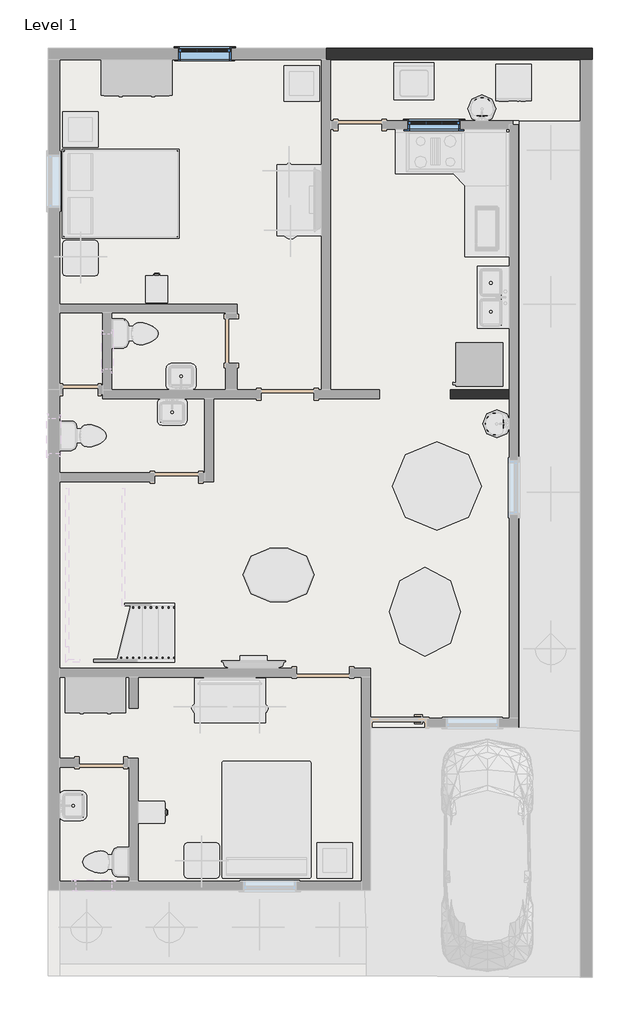
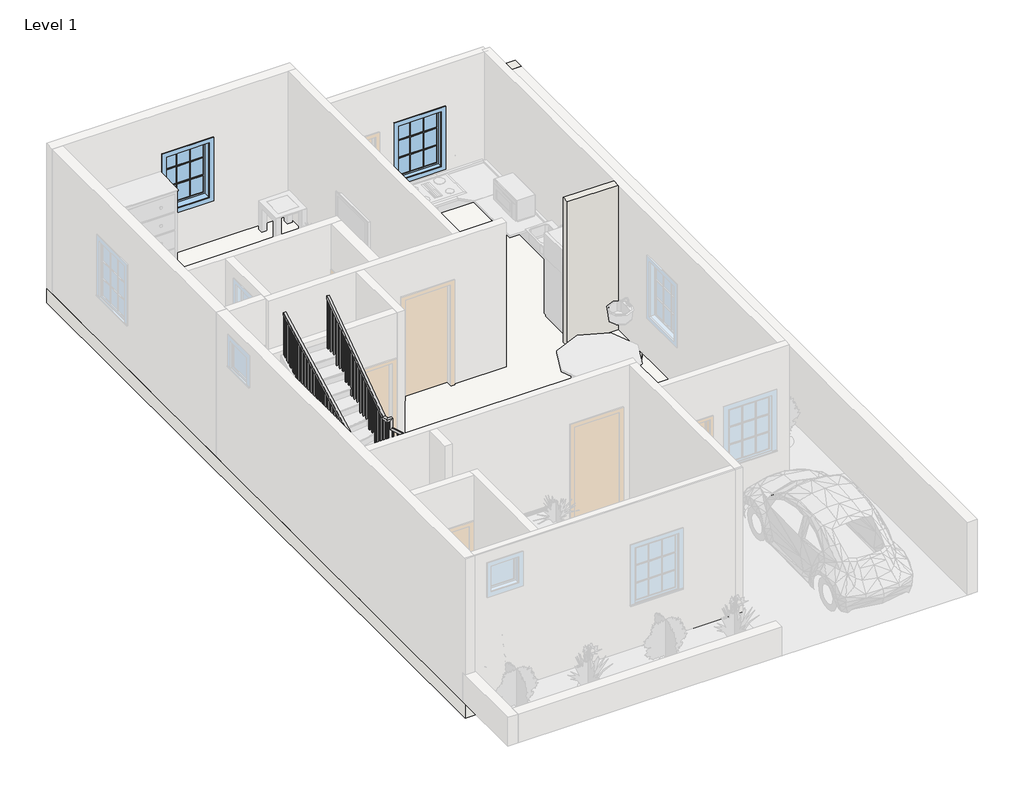
# One storey, part 2 of 3: 2 railings, 2 slabs, 2 walls, 2 windows.
"""IFC4 building model written with IfcOpenShell, lengths in millimetres."""

from ifc_helpers import new_model, si_unit, frame, origin, origin_with_axes, place, context, project, spatial, polyline, outline, extrude, faceted_brep, transform, mapped, element, save
from components import window_29c06734, window_5c190c7e

model = new_model("IFC4")

# Units and contexts
model_context = context("Model", 3, world=origin())
ifc_project = project(units=[si_unit("LENGTHUNIT", "METRE", prefix="MILLI")], contexts=[model_context])

# Site, building, storey
site = spatial("IfcSite", under=ifc_project)
building = spatial("IfcBuilding", under=site)
storey = spatial("IfcBuildingStorey", under=building, Name="Level 1", Elevation=0.0)

# Railings
placement = place(None, origin())
element("IfcRailing", 1, ObjectType="Handrail - Rectangular", at=placement, inside=storey, context=model_context, shape_type="SolidModel", body=[
    faceted_brep([(-12359.4290643, 4743.353629, 1682.9646102), (-12359.4290643, 4743.353629, 1615.1075334), (-12359.4290643, 4794.153629, 1615.1075334), (-12359.4290643, 4794.153629, 1682.9646102), (-13187.1660538, 4743.353629, 2416.0047843), (-13237.9660538, 4743.353629, 2393.1359601), (-13237.9660538, 4794.153629, 2393.1359601), (-13187.1660538, 4794.153629, 2416.0047843), (-13187.1660538, 4743.353629, 2625.457216), (-13237.9660538, 4743.353629, 2574.657216), (-13237.9660538, 4794.153629, 2574.657216), (-13187.1660538, 4794.153629, 2625.457216), (-13314.1660538, 4743.353629, 2625.457216), (-13314.1660538, 4743.353629, 2574.657216), (-13263.3660538, 4794.153629, 2574.657216), (-13263.3660538, 4794.153629, 2625.457216), (-13314.1660538, 4870.353629, 2625.457216), (-13314.1660538, 4886.3832649, 2574.657216), (-13263.3660538, 4886.3832649, 2574.657216), (-13263.3660538, 4870.353629, 2625.457216), (-13314.1660538, 6815.6906185, 3988.8904479), (-13263.3660538, 6815.6906185, 3988.8904479), (-13263.3660538, 6815.6906185, 3926.8557166), (-13314.1660538, 6815.6906185, 3926.8557166)], [[[0, 1, 2, 3]], [[1, 0, 4, 5]], [[2, 1, 5, 6]], [[3, 2, 6, 7]], [[0, 3, 7, 4]], [[5, 4, 8, 9]], [[6, 5, 9, 10]], [[7, 6, 10, 11]], [[4, 7, 11, 8]], [[9, 8, 12, 13]], [[10, 9, 13, 14]], [[11, 10, 14, 15]], [[8, 11, 15, 12]], [[13, 12, 16, 17]], [[14, 13, 17, 18]], [[15, 14, 18, 19]], [[12, 15, 19, 16]], [[20, 21, 22, 23]], [[17, 16, 20, 23]], [[18, 17, 23, 22]], [[19, 18, 22, 21]], [[16, 19, 21, 20]]]),
    extrude(outline(polyline([(6791.228629, 3909.7109805), (6810.278629, 3923.0626019), (6810.278629, 2878.6666667), (6791.228629, 2878.6666667), (6791.228629, 3909.7109805)])), frame((-13298.2910538, 0.0, 0.0), z_axis=(1.0, 0.0, 0.0), x_axis=(0.0, 1.0, 0.0)), (0.0, 0.0, 1.0), 19.05),
    extrude(outline(polyline([(6689.628629, 3838.5023328), (6708.678629, 3851.8539542), (6708.678629, 2878.6666667), (6689.628629, 2878.6666667), (6689.628629, 3838.5023328)])), frame((-13298.2910538, 0.0, 0.0), z_axis=(1.0, 0.0, 0.0), x_axis=(0.0, 1.0, 0.0)), (0.0, 0.0, 1.0), 19.05),
    extrude(outline(polyline([(6588.028629, 3767.3719643), (6607.078629, 3780.7235858), (6607.078629, 2878.6666667), (6588.028629, 2878.6666667), (6588.028629, 3767.3719643)])), frame((-13298.2910538, 0.0, 0.0), z_axis=(1.0, 0.0, 0.0), x_axis=(0.0, 1.0, 0.0)), (0.0, 0.0, 1.0), 19.05),
    extrude(outline(polyline([(6486.428629, 3696.1633166), (6505.478629, 3709.514938), (6505.478629, 2709.3333333), (6486.428629, 2709.3333333), (6486.428629, 3696.1633166)])), frame((-13298.2910538, 0.0, 0.0), z_axis=(1.0, 0.0, 0.0), x_axis=(0.0, 1.0, 0.0)), (0.0, 0.0, 1.0), 19.05),
    extrude(outline(polyline([(6384.828629, 3624.9546689), (6403.878629, 3638.3062903), (6403.878629, 2709.3333333), (6384.828629, 2709.3333333), (6384.828629, 3624.9546689)])), frame((-13298.2910538, 0.0, 0.0), z_axis=(1.0, 0.0, 0.0), x_axis=(0.0, 1.0, 0.0)), (0.0, 0.0, 1.0), 19.05),
    extrude(outline(polyline([(6283.228629, 3553.667742), (6302.278629, 3567.0193634), (6302.278629, 2709.3333333), (6283.228629, 2709.3333333), (6283.228629, 3553.667742)])), frame((-13298.2910538, 0.0, 0.0), z_axis=(1.0, 0.0, 0.0), x_axis=(0.0, 1.0, 0.0)), (0.0, 0.0, 1.0), 19.05),
    extrude(outline(polyline([(6181.628629, 3482.5373735), (6200.678629, 3495.8889949), (6200.678629, 2540.0), (6181.628629, 2540.0), (6181.628629, 3482.5373735)])), frame((-13298.2910538, 0.0, 0.0), z_axis=(1.0, 0.0, 0.0), x_axis=(0.0, 1.0, 0.0)), (0.0, 0.0, 1.0), 19.05),
    extrude(outline(polyline([(6080.028629, 3411.2504466), (6099.078629, 3424.602068), (6099.078629, 2540.0), (6080.028629, 2540.0), (6080.028629, 3411.2504466)])), frame((-13298.2910538, 0.0, 0.0), z_axis=(1.0, 0.0, 0.0), x_axis=(0.0, 1.0, 0.0)), (0.0, 0.0, 1.0), 19.05),
    extrude(outline(polyline([(5978.428629, 3340.1200781), (5997.478629, 3353.4716995), (5997.478629, 2370.6666667), (5978.428629, 2370.6666667), (5978.428629, 3340.1200781)])), frame((-13298.2910538, 0.0, 0.0), z_axis=(1.0, 0.0, 0.0), x_axis=(0.0, 1.0, 0.0)), (0.0, 0.0, 1.0), 19.05),
    extrude(outline(polyline([(5876.828629, 3268.8331511), (5895.878629, 3282.1847726), (5895.878629, 2370.6666667), (5876.828629, 2370.6666667), (5876.828629, 3268.8331511)])), frame((-13298.2910538, 0.0, 0.0), z_axis=(1.0, 0.0, 0.0), x_axis=(0.0, 1.0, 0.0)), (0.0, 0.0, 1.0), 19.05),
    extrude(outline(polyline([(5775.228629, 3197.6245034), (5794.278629, 3210.9761249), (5794.278629, 2370.6666667), (5775.228629, 2370.6666667), (5775.228629, 3197.6245034)])), frame((-13298.2910538, 0.0, 0.0), z_axis=(1.0, 0.0, 0.0), x_axis=(0.0, 1.0, 0.0)), (0.0, 0.0, 1.0), 19.05),
    extrude(outline(polyline([(5673.628629, 3126.494135), (5692.678629, 3139.8457564), (5692.678629, 2201.3333333), (5673.628629, 2201.3333333), (5673.628629, 3126.494135)])), frame((-13298.2910538, 0.0, 0.0), z_axis=(1.0, 0.0, 0.0), x_axis=(0.0, 1.0, 0.0)), (0.0, 0.0, 1.0), 19.05),
    extrude(outline(polyline([(5572.028629, 3055.207208), (5591.078629, 3068.5588295), (5591.078629, 2201.3333333), (5572.028629, 2201.3333333), (5572.028629, 3055.207208)])), frame((-13298.2910538, 0.0, 0.0), z_axis=(1.0, 0.0, 0.0), x_axis=(0.0, 1.0, 0.0)), (0.0, 0.0, 1.0), 19.05),
    extrude(outline(polyline([(5470.428629, 2983.9985603), (5489.478629, 2997.3501818), (5489.478629, 2201.3333333), (5470.428629, 2201.3333333), (5470.428629, 2983.9985603)])), frame((-13298.2910538, 0.0, 0.0), z_axis=(1.0, 0.0, 0.0), x_axis=(0.0, 1.0, 0.0)), (0.0, 0.0, 1.0), 19.05),
    extrude(outline(polyline([(5368.828629, 2912.7899126), (5387.878629, 2926.1415341), (5387.878629, 2032.0), (5368.828629, 2032.0), (5368.828629, 2912.7899126)])), frame((-13298.2910538, 0.0, 0.0), z_axis=(1.0, 0.0, 0.0), x_axis=(0.0, 1.0, 0.0)), (0.0, 0.0, 1.0), 19.05),
    extrude(outline(polyline([(5267.228629, 2841.5812649), (5286.278629, 2854.9328864), (5286.278629, 2032.0), (5267.228629, 2032.0), (5267.228629, 2841.5812649)])), frame((-13298.2910538, 0.0, 0.0), z_axis=(1.0, 0.0, 0.0), x_axis=(0.0, 1.0, 0.0)), (0.0, 0.0, 1.0), 19.05),
    extrude(outline(polyline([(5165.628629, 2770.4508964), (5184.678629, 2783.8025179), (5184.678629, 1862.6666667), (5165.628629, 1862.6666667), (5165.628629, 2770.4508964)])), frame((-13298.2910538, 0.0, 0.0), z_axis=(1.0, 0.0, 0.0), x_axis=(0.0, 1.0, 0.0)), (0.0, 0.0, 1.0), 19.05),
    extrude(outline(polyline([(5064.028629, 2699.1639695), (5083.078629, 2712.515591), (5083.078629, 1862.6666667), (5064.028629, 1862.6666667), (5064.028629, 2699.1639695)])), frame((-13298.2910538, 0.0, 0.0), z_axis=(1.0, 0.0, 0.0), x_axis=(0.0, 1.0, 0.0)), (0.0, 0.0, 1.0), 19.05),
    extrude(outline(polyline([(4962.428629, 2628.033601), (4981.478629, 2641.3852225), (4981.478629, 1693.3333333), (4962.428629, 1693.3333333), (4962.428629, 2628.033601)])), frame((-13298.2910538, 0.0, 0.0), z_axis=(1.0, 0.0, 0.0), x_axis=(0.0, 1.0, 0.0)), (0.0, 0.0, 1.0), 19.05),
    extrude(outline(polyline([(-13279.2410538, 4860.828629), (-13298.2910538, 4860.828629), (-13298.2910538, 4879.878629), (-13279.2410538, 4879.878629), (-13279.2410538, 4860.828629)])), frame((0.0, 0.0, 1693.3333333), z_axis=(0.0, 0.0, 1.0), x_axis=(1.0, 0.0, 0.0)), (0.0, 0.0, 1.0), 881.3238827),
    extrude(outline(polyline([(-13264.3040643, 4778.278629), (-13264.3040643, 4759.228629), (-13283.3540643, 4759.228629), (-13283.3540643, 4778.278629), (-13264.3040643, 4778.278629)])), frame((0.0, 0.0, 1524.0), z_axis=(0.0, 0.0, 1.0), x_axis=(1.0, 0.0, 0.0)), (0.0, 0.0, 1.0), 1050.657216),
    extrude(outline(polyline([(2326.484279, -13162.7040643), (2343.3548737, -13181.7540643), (1354.6666667, -13181.7540643), (1354.6666667, -13162.7040643), (2326.484279, -13162.7040643)])), frame((0.0, 4759.228629, 0.0), z_axis=(0.0, 1.0, 0.0), x_axis=(0.0, 0.0, 1.0)), (0.0, 0.0, 1.0), 19.05),
    extrude(outline(polyline([(2236.5077736, -13061.1040643), (2253.3783684, -13080.1540643), (1185.3333333, -13080.1540643), (1185.3333333, -13061.1040643), (2236.5077736, -13061.1040643)])), frame((0.0, 4759.228629, 0.0), z_axis=(0.0, 1.0, 0.0), x_axis=(0.0, 0.0, 1.0)), (0.0, 0.0, 1.0), 19.05),
    extrude(outline(polyline([(2146.5312682, -12959.5040643), (2163.401863, -12978.5540643), (1185.3333333, -12978.5540643), (1185.3333333, -12959.5040643), (2146.5312682, -12959.5040643)])), frame((0.0, 4759.228629, 0.0), z_axis=(0.0, 1.0, 0.0), x_axis=(0.0, 0.0, 1.0)), (0.0, 0.0, 1.0), 19.05),
    extrude(outline(polyline([(2056.5547629, -12857.9040643), (2073.4253576, -12876.9540643), (1016.0, -12876.9540643), (1016.0, -12857.9040643), (2056.5547629, -12857.9040643)])), frame((0.0, 4759.228629, 0.0), z_axis=(0.0, 1.0, 0.0), x_axis=(0.0, 0.0, 1.0)), (0.0, 0.0, 1.0), 19.05),
    extrude(outline(polyline([(1966.5782575, -12756.3040643), (1983.4488522, -12775.3540643), (1016.0, -12775.3540643), (1016.0, -12756.3040643), (1966.5782575, -12756.3040643)])), frame((0.0, 4759.228629, 0.0), z_axis=(0.0, 1.0, 0.0), x_axis=(0.0, 0.0, 1.0)), (0.0, 0.0, 1.0), 19.05),
    extrude(outline(polyline([(1876.6017521, -12654.7040643), (1893.4723469, -12673.7540643), (1016.0, -12673.7540643), (1016.0, -12654.7040643), (1876.6017521, -12654.7040643)])), frame((0.0, 4759.228629, 0.0), z_axis=(0.0, 1.0, 0.0), x_axis=(0.0, 0.0, 1.0)), (0.0, 0.0, 1.0), 19.05),
    extrude(outline(polyline([(1786.6252467, -12553.1040643), (1803.4958415, -12572.1540643), (846.6666667, -12572.1540643), (846.6666667, -12553.1040643), (1786.6252467, -12553.1040643)])), frame((0.0, 4759.228629, 0.0), z_axis=(0.0, 1.0, 0.0), x_axis=(0.0, 0.0, 1.0)), (0.0, 0.0, 1.0), 19.05),
    extrude(outline(polyline([(1696.6487414, -12451.5040643), (1713.5193361, -12470.5540643), (846.6666667, -12470.5540643), (846.6666667, -12451.5040643), (1696.6487414, -12451.5040643)])), frame((0.0, 4759.228629, 0.0), z_axis=(0.0, 1.0, 0.0), x_axis=(0.0, 0.0, 1.0)), (0.0, 0.0, 1.0), 19.05),
    extrude(outline(polyline([(-13279.2410538, 4759.228629), (-13298.2910538, 4759.228629), (-13298.2910538, 4778.278629), (-13279.2410538, 4778.278629), (-13279.2410538, 4759.228629)])), frame((0.0, 0.0, 1524.0), z_axis=(0.0, 0.0, 1.0), x_axis=(1.0, 0.0, 0.0)), (0.0, 0.0, 1.0), 1050.657216),
    extrude(outline(polyline([(6796.6406185, 3913.5040952), (6815.6906185, 3926.8557166), (6815.6906185, 2878.6666667), (6796.6406185, 2878.6666667), (6796.6406185, 3913.5040952)])), frame((-13298.2910538, 0.0, 0.0), z_axis=(1.0, 0.0, 0.0), x_axis=(0.0, 1.0, 0.0)), (0.0, 0.0, 1.0), 19.05),
    extrude(outline(polyline([(1615.1075334, -12359.4290643), (1631.9781281, -12378.4790643), (846.6666667, -12378.4790643), (846.6666667, -12359.4290643), (1615.1075334, -12359.4290643)])), frame((0.0, 4759.228629, 0.0), z_axis=(0.0, 1.0, 0.0), x_axis=(0.0, 0.0, 1.0)), (0.0, 0.0, 1.0), 19.05),
])
element("IfcRailing", 2, ObjectType="Handrail - Rectangular", at=placement, inside=storey, context=model_context, shape_type="SolidModel", body=[
    faceted_brep([(-12359.4290643, 3879.753629, 1807.8545254), (-12359.4290643, 3879.753629, 1752.3830665), (-12359.4290643, 3930.553629, 1752.3830665), (-12359.4290643, 3930.553629, 1807.8545254), (-13956.7820986, 3879.753629, 2508.4571941), (-13967.4328846, 3879.753629, 2457.6571941), (-13967.4328846, 3930.553629, 2457.6571941), (-13956.7820986, 3930.553629, 2508.4571941), (-14177.7660538, 3879.753629, 2508.4571941), (-14177.7660538, 3879.753629, 2457.6571941), (-14126.9660538, 3930.553629, 2457.6571941), (-14126.9660538, 3930.553629, 2508.4571941), (-14177.7660538, 4069.8569729, 2508.4571941), (-14177.7660538, 4082.2933675, 2457.6571941), (-14126.9660538, 4082.2933675, 2457.6571941), (-14126.9660538, 4069.8569729, 2508.4571941), (-14177.7660538, 6815.6906185, 3938.588476), (-14126.9660538, 6815.6906185, 3938.588476), (-14126.9660538, 6815.6906185, 3881.3111437), (-14177.7660538, 6815.6906185, 3881.3111437)], [[[0, 1, 2, 3]], [[1, 0, 4, 5]], [[2, 1, 5, 6]], [[3, 2, 6, 7]], [[0, 3, 7, 4]], [[5, 4, 8, 9]], [[6, 5, 9, 10]], [[7, 6, 10, 11]], [[4, 7, 11, 8]], [[9, 8, 12, 13]], [[10, 9, 13, 14]], [[11, 10, 14, 15]], [[8, 11, 15, 12]], [[16, 17, 18, 19]], [[13, 12, 16, 19]], [[14, 13, 19, 18]], [[15, 14, 18, 17]], [[12, 15, 17, 16]]]),
    extrude(outline(polyline([(6822.5819729, 3884.8947365), (6822.5819729, 2878.6666667), (6803.5319729, 2878.6666667), (6803.5319729, 3874.9727949), (6822.5819729, 3884.8947365)])), frame((-14161.8910538, 0.0, 0.0), z_axis=(1.0, 0.0, 0.0), x_axis=(0.0, 1.0, 0.0)), (0.0, 0.0, 1.0), 19.05),
    extrude(outline(polyline([(6720.9819729, 3831.9777149), (6720.9819729, 2878.6666667), (6701.9319729, 2878.6666667), (6701.9319729, 3822.0557734), (6720.9819729, 3831.9777149)])), frame((-14161.8910538, 0.0, 0.0), z_axis=(1.0, 0.0, 0.0), x_axis=(0.0, 1.0, 0.0)), (0.0, 0.0, 1.0), 19.05),
    extrude(outline(polyline([(6619.3819729, 3779.0663717), (6619.3819729, 2878.6666667), (6600.3319729, 2878.6666667), (6600.3319729, 3769.1444302), (6619.3819729, 3779.0663717)])), frame((-14161.8910538, 0.0, 0.0), z_axis=(1.0, 0.0, 0.0), x_axis=(0.0, 1.0, 0.0)), (0.0, 0.0, 1.0), 19.05),
    extrude(outline(polyline([(6517.7819729, 3726.1436718), (6517.7819729, 2709.3333333), (6498.7319729, 2709.3333333), (6498.7319729, 3716.2217303), (6517.7819729, 3726.1436718)])), frame((-14161.8910538, 0.0, 0.0), z_axis=(1.0, 0.0, 0.0), x_axis=(0.0, 1.0, 0.0)), (0.0, 0.0, 1.0), 19.05),
    extrude(outline(polyline([(6416.1819729, 3673.2266502), (6416.1819729, 2709.3333333), (6397.1319729, 2709.3333333), (6397.1319729, 3663.3047087), (6416.1819729, 3673.2266502)])), frame((-14161.8910538, 0.0, 0.0), z_axis=(1.0, 0.0, 0.0), x_axis=(0.0, 1.0, 0.0)), (0.0, 0.0, 1.0), 19.05),
    extrude(outline(polyline([(6314.5819729, 3620.315307), (6314.5819729, 2709.3333333), (6295.5319729, 2709.3333333), (6295.5319729, 3610.3933655), (6314.5819729, 3620.315307)])), frame((-14161.8910538, 0.0, 0.0), z_axis=(1.0, 0.0, 0.0), x_axis=(0.0, 1.0, 0.0)), (0.0, 0.0, 1.0), 19.05),
    extrude(outline(polyline([(6212.9819729, 3567.3926071), (6212.9819729, 2540.0), (6193.9319729, 2540.0), (6193.9319729, 3557.4706656), (6212.9819729, 3567.3926071)])), frame((-14161.8910538, 0.0, 0.0), z_axis=(1.0, 0.0, 0.0), x_axis=(0.0, 1.0, 0.0)), (0.0, 0.0, 1.0), 19.05),
    extrude(outline(polyline([(6111.3819729, 3514.4755855), (6111.3819729, 2540.0), (6092.3319729, 2540.0), (6092.3319729, 3504.553644), (6111.3819729, 3514.4755855)])), frame((-14161.8910538, 0.0, 0.0), z_axis=(1.0, 0.0, 0.0), x_axis=(0.0, 1.0, 0.0)), (0.0, 0.0, 1.0), 19.05),
    extrude(outline(polyline([(6009.7819729, 3461.558564), (6009.7819729, 2540.0), (5990.7319729, 2540.0), (5990.7319729, 3451.6366224), (6009.7819729, 3461.558564)])), frame((-14161.8910538, 0.0, 0.0), z_axis=(1.0, 0.0, 0.0), x_axis=(0.0, 1.0, 0.0)), (0.0, 0.0, 1.0), 19.05),
    extrude(outline(polyline([(5908.1819729, 3408.6415424), (5908.1819729, 2370.6666667), (5889.1319729, 2370.6666667), (5889.1319729, 3398.7196009), (5908.1819729, 3408.6415424)])), frame((-14161.8910538, 0.0, 0.0), z_axis=(1.0, 0.0, 0.0), x_axis=(0.0, 1.0, 0.0)), (0.0, 0.0, 1.0), 19.05),
    extrude(outline(polyline([(5806.5819729, 3355.7245208), (5806.5819729, 2370.6666667), (5787.5319729, 2370.6666667), (5787.5319729, 3345.8025793), (5806.5819729, 3355.7245208)])), frame((-14161.8910538, 0.0, 0.0), z_axis=(1.0, 0.0, 0.0), x_axis=(0.0, 1.0, 0.0)), (0.0, 0.0, 1.0), 19.05),
    extrude(outline(polyline([(5704.9819729, 3302.8131776), (5704.9819729, 2370.6666667), (5685.9319729, 2370.6666667), (5685.9319729, 3292.8912361), (5704.9819729, 3302.8131776)])), frame((-14161.8910538, 0.0, 0.0), z_axis=(1.0, 0.0, 0.0), x_axis=(0.0, 1.0, 0.0)), (0.0, 0.0, 1.0), 19.05),
    extrude(outline(polyline([(5603.3819729, 3249.8961561), (5603.3819729, 2201.3333333), (5584.3319729, 2201.3333333), (5584.3319729, 3239.9742145), (5603.3819729, 3249.8961561)])), frame((-14161.8910538, 0.0, 0.0), z_axis=(1.0, 0.0, 0.0), x_axis=(0.0, 1.0, 0.0)), (0.0, 0.0, 1.0), 19.05),
    extrude(outline(polyline([(5501.7819729, 3196.9791345), (5501.7819729, 2201.3333333), (5482.7319729, 2201.3333333), (5482.7319729, 3187.057193), (5501.7819729, 3196.9791345)])), frame((-14161.8910538, 0.0, 0.0), z_axis=(1.0, 0.0, 0.0), x_axis=(0.0, 1.0, 0.0)), (0.0, 0.0, 1.0), 19.05),
    extrude(outline(polyline([(5400.1819729, 3144.062113), (5400.1819729, 2201.3333333), (5381.1319729, 2201.3333333), (5381.1319729, 3134.1401714), (5400.1819729, 3144.062113)])), frame((-14161.8910538, 0.0, 0.0), z_axis=(1.0, 0.0, 0.0), x_axis=(0.0, 1.0, 0.0)), (0.0, 0.0, 1.0), 19.05),
    extrude(outline(polyline([(5298.5819729, 3091.1450914), (5298.5819729, 2032.0), (5279.5319729, 2032.0), (5279.5319729, 3081.2231498), (5298.5819729, 3091.1450914)])), frame((-14161.8910538, 0.0, 0.0), z_axis=(1.0, 0.0, 0.0), x_axis=(0.0, 1.0, 0.0)), (0.0, 0.0, 1.0), 19.05),
    extrude(outline(polyline([(5196.9819729, 3038.2280698), (5196.9819729, 2032.0), (5177.9319729, 2032.0), (5177.9319729, 3028.3061283), (5196.9819729, 3038.2280698)])), frame((-14161.8910538, 0.0, 0.0), z_axis=(1.0, 0.0, 0.0), x_axis=(0.0, 1.0, 0.0)), (0.0, 0.0, 1.0), 19.05),
    extrude(outline(polyline([(5095.3819729, 2985.3110483), (5095.3819729, 2032.0), (5076.3319729, 2032.0), (5076.3319729, 2975.3891067), (5095.3819729, 2985.3110483)])), frame((-14161.8910538, 0.0, 0.0), z_axis=(1.0, 0.0, 0.0), x_axis=(0.0, 1.0, 0.0)), (0.0, 0.0, 1.0), 19.05),
    extrude(outline(polyline([(4993.7819729, 2932.3940267), (4993.7819729, 1862.6666667), (4974.7319729, 1862.6666667), (4974.7319729, 2922.4720852), (4993.7819729, 2932.3940267)])), frame((-14161.8910538, 0.0, 0.0), z_axis=(1.0, 0.0, 0.0), x_axis=(0.0, 1.0, 0.0)), (0.0, 0.0, 1.0), 19.05),
    extrude(outline(polyline([(4892.1819729, 2879.4770051), (4892.1819729, 1862.6666667), (4873.1319729, 1862.6666667), (4873.1319729, 2869.5550636), (4892.1819729, 2879.4770051)])), frame((-14161.8910538, 0.0, 0.0), z_axis=(1.0, 0.0, 0.0), x_axis=(0.0, 1.0, 0.0)), (0.0, 0.0, 1.0), 19.05),
    extrude(outline(polyline([(4790.5819729, 2826.5599836), (4790.5819729, 1862.6666667), (4771.5319729, 1862.6666667), (4771.5319729, 2816.638042), (4790.5819729, 2826.5599836)])), frame((-14161.8910538, 0.0, 0.0), z_axis=(1.0, 0.0, 0.0), x_axis=(0.0, 1.0, 0.0)), (0.0, 0.0, 1.0), 19.05),
    extrude(outline(polyline([(4688.9819729, 2773.642962), (4688.9819729, 1693.3333333), (4669.9319729, 1693.3333333), (4669.9319729, 2763.7210205), (4688.9819729, 2773.642962)])), frame((-14161.8910538, 0.0, 0.0), z_axis=(1.0, 0.0, 0.0), x_axis=(0.0, 1.0, 0.0)), (0.0, 0.0, 1.0), 19.05),
    extrude(outline(polyline([(4587.3819729, 2720.7259404), (4587.3819729, 1693.3333333), (4568.3319729, 1693.3333333), (4568.3319729, 2710.8039989), (4587.3819729, 2720.7259404)])), frame((-14161.8910538, 0.0, 0.0), z_axis=(1.0, 0.0, 0.0), x_axis=(0.0, 1.0, 0.0)), (0.0, 0.0, 1.0), 19.05),
    extrude(outline(polyline([(4485.7819729, 2667.8089189), (4485.7819729, 1693.3333333), (4466.7319729, 1693.3333333), (4466.7319729, 2657.8869773), (4485.7819729, 2667.8089189)])), frame((-14161.8910538, 0.0, 0.0), z_axis=(1.0, 0.0, 0.0), x_axis=(0.0, 1.0, 0.0)), (0.0, 0.0, 1.0), 19.05),
    extrude(outline(polyline([(4384.1819729, 2614.8918973), (4384.1819729, 1693.3333333), (4365.1319729, 1693.3333333), (4365.1319729, 2604.9699558), (4384.1819729, 2614.8918973)])), frame((-14161.8910538, 0.0, 0.0), z_axis=(1.0, 0.0, 0.0), x_axis=(0.0, 1.0, 0.0)), (0.0, 0.0, 1.0), 19.05),
    extrude(outline(polyline([(4282.5819729, 2561.9748757), (4282.5819729, 1524.0), (4263.5319729, 1524.0), (4263.5319729, 2552.0529342), (4282.5819729, 2561.9748757)])), frame((-14161.8910538, 0.0, 0.0), z_axis=(1.0, 0.0, 0.0), x_axis=(0.0, 1.0, 0.0)), (0.0, 0.0, 1.0), 19.05),
    extrude(outline(polyline([(4180.9819729, 2509.0578542), (4180.9819729, 1524.0), (4161.9319729, 1524.0), (4161.9319729, 2499.1359126), (4180.9819729, 2509.0578542)])), frame((-14161.8910538, 0.0, 0.0), z_axis=(1.0, 0.0, 0.0), x_axis=(0.0, 1.0, 0.0)), (0.0, 0.0, 1.0), 19.05),
    extrude(outline(polyline([(-14161.8910538, 3997.228629), (-14161.8910538, 4016.278629), (-14142.8410538, 4016.278629), (-14142.8410538, 3997.228629), (-14161.8910538, 3997.228629)])), frame((0.0, 0.0, 1524.0), z_axis=(0.0, 0.0, 1.0), x_axis=(1.0, 0.0, 0.0)), (0.0, 0.0, 1.0), 933.6571941),
    extrude(outline(polyline([(-14048.8570986, 3895.628629), (-14067.9070986, 3895.628629), (-14067.9070986, 3914.678629), (-14048.8570986, 3914.678629), (-14048.8570986, 3895.628629)])), frame((0.0, 0.0, 1524.0), z_axis=(0.0, 0.0, 1.0), x_axis=(1.0, 0.0, 0.0)), (0.0, 0.0, 1.0), 933.6571941),
    extrude(outline(polyline([(2424.9906144, -13892.9540643), (1524.0, -13892.9540643), (1524.0, -13873.9040643), (2416.6352411, -13873.9040643), (2424.9906144, -13892.9540643)])), frame((0.0, 3895.628629, 0.0), z_axis=(0.0, 1.0, 0.0), x_axis=(0.0, 0.0, 1.0)), (0.0, 0.0, 1.0), 19.05),
    extrude(outline(polyline([(2380.4286236, -13791.3540643), (1524.0, -13791.3540643), (1524.0, -13772.3040643), (2372.0732504, -13772.3040643), (2380.4286236, -13791.3540643)])), frame((0.0, 3895.628629, 0.0), z_axis=(0.0, 1.0, 0.0), x_axis=(0.0, 0.0, 1.0)), (0.0, 0.0, 1.0), 19.05),
    extrude(outline(polyline([(2335.8666329, -13689.7540643), (1354.6666667, -13689.7540643), (1354.6666667, -13670.7040643), (2327.5112596, -13670.7040643), (2335.8666329, -13689.7540643)])), frame((0.0, 3895.628629, 0.0), z_axis=(0.0, 1.0, 0.0), x_axis=(0.0, 0.0, 1.0)), (0.0, 0.0, 1.0), 19.05),
    extrude(outline(polyline([(2291.3046421, -13588.1540643), (1354.6666667, -13588.1540643), (1354.6666667, -13569.1040643), (2282.9492689, -13569.1040643), (2291.3046421, -13588.1540643)])), frame((0.0, 3895.628629, 0.0), z_axis=(0.0, 1.0, 0.0), x_axis=(0.0, 0.0, 1.0)), (0.0, 0.0, 1.0), 19.05),
    extrude(outline(polyline([(2246.7426514, -13486.5540643), (1354.6666667, -13486.5540643), (1354.6666667, -13467.5040643), (2238.3872781, -13467.5040643), (2246.7426514, -13486.5540643)])), frame((0.0, 3895.628629, 0.0), z_axis=(0.0, 1.0, 0.0), x_axis=(0.0, 0.0, 1.0)), (0.0, 0.0, 1.0), 19.05),
    extrude(outline(polyline([(2202.1806606, -13384.9540643), (1354.6666667, -13384.9540643), (1354.6666667, -13365.9040643), (2193.8252874, -13365.9040643), (2202.1806606, -13384.9540643)])), frame((0.0, 3895.628629, 0.0), z_axis=(0.0, 1.0, 0.0), x_axis=(0.0, 0.0, 1.0)), (0.0, 0.0, 1.0), 19.05),
    extrude(outline(polyline([(2157.6186699, -13283.3540643), (1185.3333333, -13283.3540643), (1185.3333333, -13264.3040643), (2149.2632966, -13264.3040643), (2157.6186699, -13283.3540643)])), frame((0.0, 3895.628629, 0.0), z_axis=(0.0, 1.0, 0.0), x_axis=(0.0, 0.0, 1.0)), (0.0, 0.0, 1.0), 19.05),
    extrude(outline(polyline([(2113.0566791, -13181.7540643), (1185.3333333, -13181.7540643), (1185.3333333, -13162.7040643), (2104.7013059, -13162.7040643), (2113.0566791, -13181.7540643)])), frame((0.0, 3895.628629, 0.0), z_axis=(0.0, 1.0, 0.0), x_axis=(0.0, 0.0, 1.0)), (0.0, 0.0, 1.0), 19.05),
    extrude(outline(polyline([(2068.4946884, -13080.1540643), (1185.3333333, -13080.1540643), (1185.3333333, -13061.1040643), (2060.1393151, -13061.1040643), (2068.4946884, -13080.1540643)])), frame((0.0, 3895.628629, 0.0), z_axis=(0.0, 1.0, 0.0), x_axis=(0.0, 0.0, 1.0)), (0.0, 0.0, 1.0), 19.05),
    extrude(outline(polyline([(2023.9326976, -12978.5540643), (1185.3333333, -12978.5540643), (1185.3333333, -12959.5040643), (2015.5773244, -12959.5040643), (2023.9326976, -12978.5540643)])), frame((0.0, 3895.628629, 0.0), z_axis=(0.0, 1.0, 0.0), x_axis=(0.0, 0.0, 1.0)), (0.0, 0.0, 1.0), 19.05),
    extrude(outline(polyline([(1979.3707069, -12876.9540643), (1016.0, -12876.9540643), (1016.0, -12857.9040643), (1971.0153336, -12857.9040643), (1979.3707069, -12876.9540643)])), frame((0.0, 3895.628629, 0.0), z_axis=(0.0, 1.0, 0.0), x_axis=(0.0, 0.0, 1.0)), (0.0, 0.0, 1.0), 19.05),
    extrude(outline(polyline([(1934.8087161, -12775.3540643), (1016.0, -12775.3540643), (1016.0, -12756.3040643), (1926.4533429, -12756.3040643), (1934.8087161, -12775.3540643)])), frame((0.0, 3895.628629, 0.0), z_axis=(0.0, 1.0, 0.0), x_axis=(0.0, 0.0, 1.0)), (0.0, 0.0, 1.0), 19.05),
    extrude(outline(polyline([(1890.2467254, -12673.7540643), (1016.0, -12673.7540643), (1016.0, -12654.7040643), (1881.8913521, -12654.7040643), (1890.2467254, -12673.7540643)])), frame((0.0, 3895.628629, 0.0), z_axis=(0.0, 1.0, 0.0), x_axis=(0.0, 0.0, 1.0)), (0.0, 0.0, 1.0), 19.05),
    extrude(outline(polyline([(1845.6847346, -12572.1540643), (846.6666667, -12572.1540643), (846.6666667, -12553.1040643), (1837.3293614, -12553.1040643), (1845.6847346, -12572.1540643)])), frame((0.0, 3895.628629, 0.0), z_axis=(0.0, 1.0, 0.0), x_axis=(0.0, 0.0, 1.0)), (0.0, 0.0, 1.0), 19.05),
    extrude(outline(polyline([(1801.1227439, -12470.5540643), (846.6666667, -12470.5540643), (846.6666667, -12451.5040643), (1792.7673706, -12451.5040643), (1801.1227439, -12470.5540643)])), frame((0.0, 3895.628629, 0.0), z_axis=(0.0, 1.0, 0.0), x_axis=(0.0, 0.0, 1.0)), (0.0, 0.0, 1.0), 19.05),
    extrude(outline(polyline([(-14161.8910538, 4060.3319729), (-14161.8910538, 4079.3819729), (-14142.8410538, 4079.3819729), (-14142.8410538, 4060.3319729), (-14161.8910538, 4060.3319729)])), frame((0.0, 0.0, 1524.0), z_axis=(0.0, 0.0, 1.0), x_axis=(1.0, 0.0, 0.0)), (0.0, 0.0, 1.0), 933.6571941),
    extrude(outline(polyline([(-14142.8410538, 3895.628629), (-14161.8910538, 3895.628629), (-14161.8910538, 3914.678629), (-14142.8410538, 3914.678629), (-14142.8410538, 3895.628629)])), frame((0.0, 0.0, 1524.0), z_axis=(0.0, 0.0, 1.0), x_axis=(1.0, 0.0, 0.0)), (0.0, 0.0, 1.0), 933.6571941),
    extrude(outline(polyline([(2457.1634218, -13966.3070986), (1524.0, -13966.3070986), (1524.0, -13947.2570986), (2448.8080486, -13947.2570986), (2457.1634218, -13966.3070986)])), frame((0.0, 3895.628629, 0.0), z_axis=(0.0, 1.0, 0.0), x_axis=(0.0, 0.0, 1.0)), (0.0, 0.0, 1.0), 19.05),
    extrude(outline(polyline([(6815.6906185, 3881.3111437), (6815.6906185, 2878.6666667), (6796.6406185, 2878.6666667), (6796.6406185, 3871.3892021), (6815.6906185, 3881.3111437)])), frame((-14161.8910538, 0.0, 0.0), z_axis=(1.0, 0.0, 0.0), x_axis=(0.0, 1.0, 0.0)), (0.0, 0.0, 1.0), 19.05),
    extrude(outline(polyline([(1760.7384398, -12378.4790643), (846.6666667, -12378.4790643), (846.6666667, -12359.4290643), (1752.3830665, -12359.4290643), (1760.7384398, -12378.4790643)])), frame((0.0, 3895.628629, 0.0), z_axis=(0.0, 1.0, 0.0), x_axis=(0.0, 0.0, 1.0)), (0.0, 0.0, 1.0), 19.05),
])

# Slabs
element("IfcSlab", 3, ObjectType="Generic - 12\"", at=placement, inside=storey, context=model_context, shape_type="SweptSolid", body=[
    extrude(outline(polyline([(-9681.9660538, 14369.953629), (-9681.9660538, 14166.753629), (-9681.9660538, 13125.353629), (-6519.6660538, 13125.353629), (-6443.4660538, 13125.353629), (-6443.4660538, 2711.353629), (-8996.1660538, 2711.353629), (-8996.1660538, -82.646371), (-14533.3660538, -82.646371), (-14533.3660538, 14369.953629), (-9681.9660538, 14369.953629)])), frame((0.0, 0.0, -304.8), z_axis=(0.0, 0.0, 1.0), x_axis=(1.0, 0.0, 0.0)), (0.0, 0.0, 1.0), 304.8),
])
element("IfcSlab", 4, ObjectType="Generic - 12\"", at=placement, inside=storey, context=model_context, shape_type="SweptSolid", body=[
    extrude(outline(polyline([(-5287.7660538, 14369.953629), (-5287.7660538, 13125.353629), (-9758.1660538, 13125.353629), (-9758.1660538, 14369.953629), (-5287.7660538, 14369.953629)])), frame((0.0, 0.0, -304.8), z_axis=(0.0, 0.0, 1.0), x_axis=(1.0, 0.0, 0.0)), (0.0, 0.0, 1.0), 304.8),
])

# Walls
element("IfcWall", 5, ObjectType="Generic - 8\" 2", at=placement, inside=storey, context=model_context, shape_type="Brep", body=[
    faceted_brep([(-9758.1660538, 14166.753629, 0.0), (-9681.9660538, 14166.753629, 0.0), (-5389.3660538, 14166.753629, 0.0), (-5186.1660538, 14166.753629, 0.0), (-5186.1660538, 14166.753629, 1524.0), (-5389.3660538, 14166.753629, 1524.0), (-9758.1660538, 14166.753629, 1524.0), (-9758.1660538, 14369.953629, 0.0), (-9758.1660538, 14369.953629, 1524.0), (-5186.1660538, 14369.953629, 1524.0), (-5186.1660538, 14369.953629, 0.0)], [[[0, 1, 2, 3, 4, 5, 6]], [[7, 8, 9, 10]], [[3, 2, 1, 0, 7, 10]], [[6, 5, 4, 9, 8]], [[0, 6, 8, 7]], [[4, 3, 10, 9]]]),
])
element("IfcWall", 6, ObjectType="INNER 6\"", at=placement, inside=storey, context=model_context, shape_type="SweptSolid", body=[
    extrude(outline(polyline([(-7624.5660538, 8502.553629), (-6608.5660538, 8502.553629), (-6608.5660538, 8350.153629), (-7624.5660538, 8350.153629), (-7624.5660538, 8502.553629)])), origin_with_axes(), (0.0, 0.0, 1.0), 3048.0),
])

# Windows
window_shape = window_29c06734(model_context)
element("IfcWindow", 7, ObjectType="Casement 3x3 with Trim : 36\" x 48\"", at=placement, inside=storey, context=model_context, shape_type="MappedRepresentation", body=[
    mapped(window_shape, transform((-11840.9660538, 14268.353629, 0.0), x_axis=(1.0, 0.0, 0.0), y_axis=(0.0, 1.0, 0.0), z_axis=(0.0, 0.0, 1.0))),
])
window_2_shape = window_5c190c7e(model_context)
element("IfcWindow", 8, ObjectType="Casement 3x3 with Trim : 36\" x 48\"", at=placement, inside=storey, context=model_context, shape_type="MappedRepresentation", body=[
    mapped(window_2_shape, transform((-7903.9660538, 13049.153629, 0.0), x_axis=(1.0, 0.0, 0.0), y_axis=(0.0, 1.0, 0.0), z_axis=(0.0, 0.0, 1.0))),
])

save(model, "model.ifc")

# Revit data of these elements
# Type "Handrail - Rectangular"
#   Assembly Code = "C2010400"
#   built-in parameter 1008612 = 0.0416667 (stored number, unit not read)
#   built-in parameter 1008611 = 0.0416667 (stored number, unit not read)
#   built-in parameter 1008609 = 0.333333 (stored number, unit not read)
#   built-in parameter 1008604 = 0.166667 (stored number, unit not read)
#   built-in parameter 1008603 = 0.166667 (stored number, unit not read)
#   Railing Height = 3' - 0"
#   built-in parameter 1008630 = 2
#   built-in parameter 1008610 = 2
#   built-in parameter 1008618 = Baluster - Square : 3/4"
# Type "Generic - 12\""
#   Assembly Code = "B1010"
#   Function = 0
#   Layers, outside or top first: 1' - 0" no material (function 1)
# Type "Generic - 8\" 2"
#   Assembly Code = "B2010"
#   Layers, outside or top first: 0' - 8" "Birch" (function 1)
# Type "INNER 6\""
#   Assembly Code = "B2010"
#   Layers, outside or top first: 0' - 6" "Brick, Common" (function 1)
# Type "Casement 3x3 with Trim : 36\" x 48\""
#   Type Mark = "10"
#   Construction Type Id = "GSP4R"
#   Assembly Code = "B2020100"
#   Analytic Construction = "1/8 in Pilkington single glazing"
#   Visual Light Transmittance = 0.9
#   Solar Heat Gain Coefficient = 0.78
#   Heat Transfer Coefficient (U) = 0.6496 BTU/(h·ft²·°F)
#   Height = 4' - 0"
#   Default Sill Height = 3' - 0"
#   Trim Projection - Ext. = 0' - 0 1/2"
#   Trim Projection - Int. = 0' - 0 3/4"
#   Trim Width - Exterior = 0' - 3 1/2"
#   Trim Width - Interior = 0' - 3 1/2"
#   Width = 3' - 0"
#   Window Inset = 0' - 0 3/4"
#   Define Thermal Properties by = 1
#   Glass Pane Material = Glass
#   Sash Material = Sash
#   Trim Exterior Material = Trim
#   Trim Interior Material = Trim
#   Wall Closure = (empty or 0)
# Elements 1, 2 (IfcRailing, "Handrail - Rectangular")
#   Phase Created = New Construction
# Elements 3, 4 (IfcSlab, "Generic - 12\"")
#   Height Offset From Level = 0' - 0"
#   Phase Created = New Construction
#   Materials on its faces: "Default Floor"
# Element 5 (IfcWall, "Generic - 8\" 2")
#   Top Offset = 0' - 0"
#   Base Offset = 0' - 0"
#   Unconnected Height = 5' - 0"
#   wall height = 5' - 0"
#   Phase Created = New Construction
#   Base Constraint = Level 1
#   Materials on its faces: "Birch"
# Element 6 (IfcWall, "INNER 6\"")
#   Top Offset = 0' - 0"
#   Base Offset = 0' - 0"
#   Unconnected Height = 10' - 0"
#   wall height = 10' - 0"
#   Phase Created = New Construction
#   Base Constraint = Level 1
#   Materials on its faces: "Brick, Common"
# Element 7 (IfcWindow, "Casement 3x3 with Trim : 36\" x 48\"")
#   Mark = "2"
#   Phase Created = New Construction
#   Materials on its faces: "Sash", "Glass", "Trim"
# Element 8 (IfcWindow, "Casement 3x3 with Trim : 36\" x 48\"")
#   Mark = "4"
#   Phase Created = New Construction
#   Materials on its faces: "Sash", "Glass", "Trim"
# Materials
#   "Birch": class "Wood", colour RGB 224 178 126, transparency 0, Description = "Betula Alleghaniensis", Cost = 0
#   "Brick, Common": class "Masonry", colour RGB 170 98 104, transparency 0, Description = "Common brick", Cost = 0
#   "Glass": class "Glass", colour RGB 0 128 192, transparency 0.75, Description = "Soda Lime Glass", Cost = 0
#   "Sash": class "Wood", colour RGB 224 178 126, transparency 0
#   "Trim": class "Wood", colour RGB 224 178 126, transparency 0
#   "Default Floor": colour RGB 128 128 128, transparency 0
